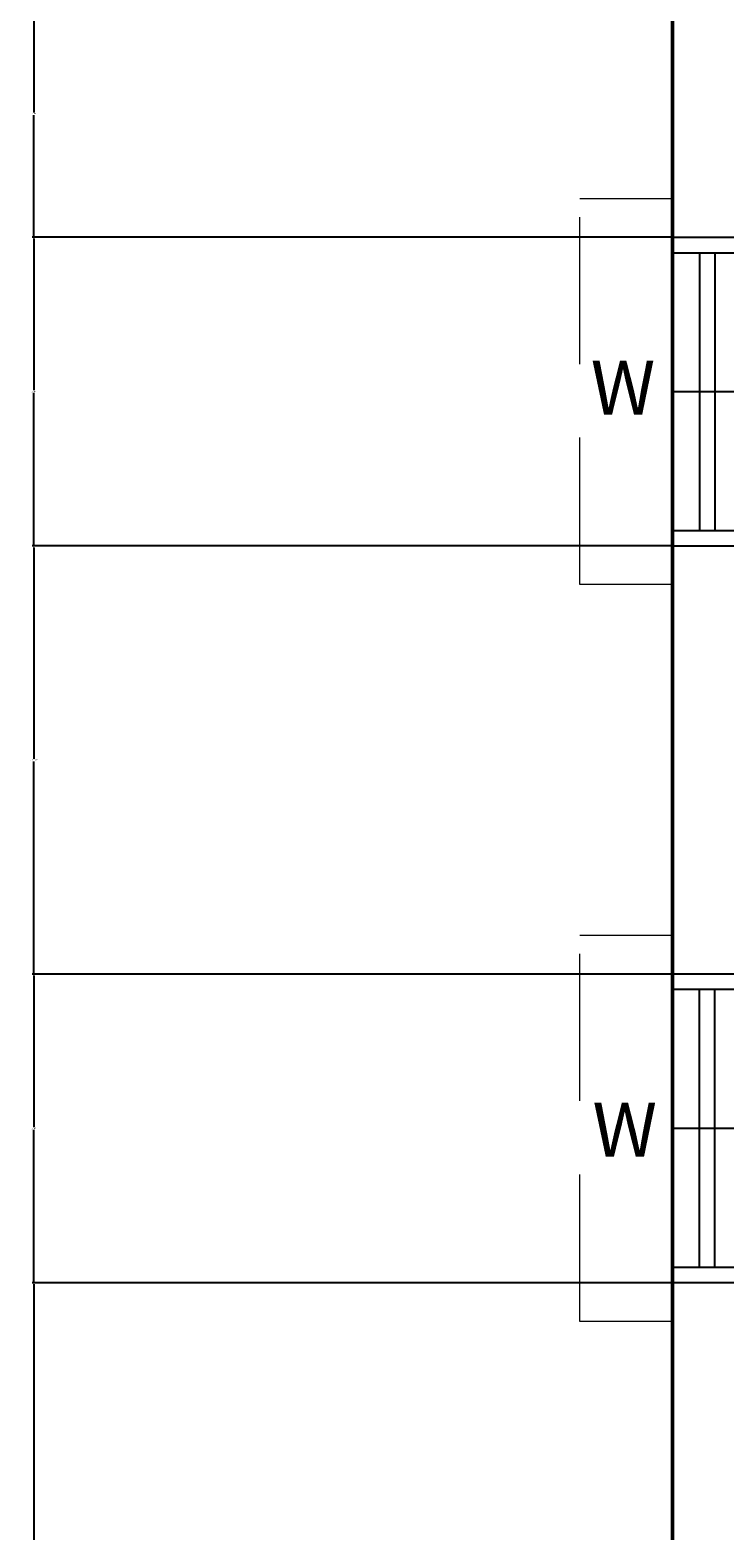
# Model space of a CAD drawing. Units: inches. Extents: x 37 to 824, y -700 to 234.
# Tile 27 of 77: x 78 to 168, y -269 to -75. Entities that reach past the tile are written whole.
import ezdxf

# ---------------------------------------------------------------- set-up
doc = ezdxf.new("R2010")
doc.units = ezdxf.units.IN
doc.header["$MEASUREMENT"] = 0
doc.linetypes.add('DASHED', pattern=[19.05, 12.7, -6.35])
for name, color, linetype, lineweight in [('A-ANNO-DIMS', 2, 'Continuous', 18), ('A-ANNO-TEXT', 7, 'Continuous', 18), ('A-GLAZ', 4, 'Continuous', 25), ('A-ROOF-OVHD', 1, 'DASHED', 18), ('A-WALL', 2, 'Continuous', 50)]:
    doc.layers.add(name, color=color, linetype=linetype, lineweight=lineweight)
doc.styles.get("Standard").update_dxf_attribs({"font": 'arial.ttf'})
doc.dimstyles.get("Standard").update_dxf_attribs({"dimtxt": 0.18, "dimasz": 0.18, "dimexe": 0.18, "dimexo": 0.0625, "dimgap": 0.09, "dimtad": 0, "dimtih": 1, "dimtoh": 1, "dimdec": 1, "dimzin": 0, "dimdsep": 46, "dimlunit": 4, "dimtxsty": 'Standard', "dimcen": 0.09, "dimadec": 0, "dimazin": 0, "dimtfac": 1, "dimtdec": 1, "dimtofl": 0, "dimtmove": 0, "dimatfit": 3, "dimfxl": 1, "dimtolj": 1, "dimtzin": 0, "dimarcsym": 0})

# ---------------------------------------------------------------- blocks, each defined once
blk = doc.blocks.new('WIN-900')
for p, q in [((0, 9), (0, 0)), ((2, 9), (2, 0)), ((20, 9), (20, 0)), ((38, 9), (38, 0)), ((40, 9), (40, 0)), ((38, 5.5), (2, 5.5)), ((38, 3.5), (2, 3.5))]:
    blk.add_line(p, q)
blk = doc.blocks.new('*D55')
at = {"layer": 'A-ANNO-DIMS', "color": 0, "lineweight": -2, "ltscale": 0.5, "transparency": 16777216}
for p, q in [((161.01, -69.41), (78.16, -69.41)), ((78.34, -69.59), (78.34, -85.23)), ((78.34, -101.23), (78.34, -85.59)), ((161.01, -101.41), (78.16, -101.41))]:
    blk.add_line(p, q, dxfattribs=at)
at = {"layer": 'A-ANNO-DIMS', "color": 0, "ltscale": 0.5, "transparency": 16777216}
for points in [[(78.31, -69.59), (78.37, -69.59), (78.34, -69.41)], [(78.31, -101.23), (78.37, -101.23), (78.34, -101.41)]]:
    blk.add_solid(points, dxfattribs=at)
at = {"layer": 'Defpoints', "color": 0, "ltscale": 0.5, "transparency": 16777216}
for p in [(161.08, -69.41), (78.34, -101.41), (161.08, -101.41)]:
    blk.add_point(p, dxfattribs=at)
at = {"layer": 'A-ANNO-DIMS', "color": 0, "ltscale": 0.5, "transparency": 16777216, "insert": (78.34, -85.41), "char_height": 0.18, "attachment_point": 5}
blk.add_mtext('\\A1;2\'-8"', dxfattribs=at)
blk = doc.blocks.new('*D56')
at = {"layer": 'A-ANNO-DIMS', "color": 0, "lineweight": -2, "ltscale": 0.5, "transparency": 16777216}
for p, q in [((161.01, -101.41), (78.16, -101.41)), ((78.34, -101.59), (78.34, -121.23)), ((78.34, -141.23), (78.34, -121.59)), ((161.01, -141.41), (78.16, -141.41))]:
    blk.add_line(p, q, dxfattribs=at)
at = {"layer": 'A-ANNO-DIMS', "color": 0, "ltscale": 0.5, "transparency": 16777216}
for points in [[(78.31, -101.59), (78.37, -101.59), (78.34, -101.41)], [(78.31, -141.23), (78.37, -141.23), (78.34, -141.41)]]:
    blk.add_solid(points, dxfattribs=at)
at = {"layer": 'Defpoints', "color": 0, "ltscale": 0.5, "transparency": 16777216}
for p in [(161.08, -101.41), (78.34, -141.41), (161.08, -141.41)]:
    blk.add_point(p, dxfattribs=at)
at = {"layer": 'A-ANNO-DIMS', "color": 0, "ltscale": 0.5, "transparency": 16777216, "insert": (78.34, -121.41), "char_height": 0.18, "attachment_point": 5}
blk.add_mtext('\\A1;3\'-4"', dxfattribs=at)
blk = doc.blocks.new('*D57')
at = {"layer": 'A-ANNO-DIMS', "color": 0, "lineweight": -2, "ltscale": 0.5, "transparency": 16777216}
for p, q in [((161.01, -141.41), (78.16, -141.41)), ((78.34, -141.59), (78.34, -168.98)), ((78.34, -196.73), (78.34, -169.34)), ((161.01, -196.91), (78.16, -196.91))]:
    blk.add_line(p, q, dxfattribs=at)
at = {"layer": 'A-ANNO-DIMS', "color": 0, "ltscale": 0.5, "transparency": 16777216}
for points in [[(78.31, -141.59), (78.37, -141.59), (78.34, -141.41)], [(78.31, -196.73), (78.37, -196.73), (78.34, -196.91)]]:
    blk.add_solid(points, dxfattribs=at)
at = {"layer": 'Defpoints', "color": 0, "ltscale": 0.5, "transparency": 16777216}
for p in [(161.08, -141.41), (78.34, -196.91), (161.08, -196.91)]:
    blk.add_point(p, dxfattribs=at)
at = {"layer": 'A-ANNO-DIMS', "color": 0, "ltscale": 0.5, "transparency": 16777216, "insert": (78.34, -169.16), "char_height": 0.18, "attachment_point": 5}
blk.add_mtext('\\A1;4\'-7 1/2"', dxfattribs=at)
blk = doc.blocks.new('*D58')
at = {"layer": 'A-ANNO-DIMS', "color": 0, "lineweight": -2, "ltscale": 0.5, "transparency": 16777216}
for p, q in [((161.01, -196.91), (78.16, -196.91)), ((78.34, -197.09), (78.34, -216.73)), ((78.34, -236.73), (78.34, -217.09)), ((161.01, -236.91), (78.16, -236.91))]:
    blk.add_line(p, q, dxfattribs=at)
at = {"layer": 'A-ANNO-DIMS', "color": 0, "ltscale": 0.5, "transparency": 16777216}
for points in [[(78.31, -197.09), (78.37, -197.09), (78.34, -196.91)], [(78.31, -236.73), (78.37, -236.73), (78.34, -236.91)]]:
    blk.add_solid(points, dxfattribs=at)
at = {"layer": 'Defpoints', "color": 0, "ltscale": 0.5, "transparency": 16777216}
for p in [(161.08, -196.91), (78.34, -236.91), (161.08, -236.91)]:
    blk.add_point(p, dxfattribs=at)
at = {"layer": 'A-ANNO-DIMS', "color": 0, "ltscale": 0.5, "transparency": 16777216, "insert": (78.34, -216.91), "char_height": 0.18, "attachment_point": 5}
blk.add_mtext('\\A1;3\'-4"', dxfattribs=at)
blk = doc.blocks.new('*D59')
at = {"layer": 'A-ANNO-DIMS', "color": 0, "lineweight": -2, "ltscale": 0.5, "transparency": 16777216}
for p, q in [((161.01, -236.91), (78.16, -236.91)), ((78.34, -237.09), (78.34, -301.23)), ((78.34, -365.73), (78.34, -301.59)), ((161.01, -365.91), (78.16, -365.91))]:
    blk.add_line(p, q, dxfattribs=at)
at = {"layer": 'A-ANNO-DIMS', "color": 0, "ltscale": 0.5, "transparency": 16777216}
for points in [[(78.31, -237.09), (78.37, -237.09), (78.34, -236.91)], [(78.31, -365.73), (78.37, -365.73), (78.34, -365.91)]]:
    blk.add_solid(points, dxfattribs=at)
at = {"layer": 'Defpoints', "color": 0, "ltscale": 0.5, "transparency": 16777216}
for p in [(161.08, -236.91), (78.34, -365.91), (161.08, -365.91)]:
    blk.add_point(p, dxfattribs=at)
at = {"layer": 'A-ANNO-DIMS', "color": 0, "ltscale": 0.5, "transparency": 16777216, "insert": (78.34, -301.41), "char_height": 0.18, "attachment_point": 5}
blk.add_mtext('\\A1;10\'-9"', dxfattribs=at)

msp = doc.modelspace()

# ---------------------------------------------------------------- linework, layer by layer
at = {"layer": 'A-ROOF-OVHD', "ltscale": 1.5}
for p, q in [((161.08, -96.41), (149.08, -96.41)), ((149.08, -146.41), (149.08, -96.41)), ((161.08, -101.41), (161.08, -96.41)), ((161.08, -141.41), (161.08, -146.41)), ((161.08, -146.41), (149.08, -146.41)), ((161.08, -191.91), (149.08, -191.91)), ((149.08, -241.91), (149.08, -191.91)), ((161.08, -196.91), (161.08, -191.91)), ((161.08, -236.91), (161.08, -241.91)), ((161.08, -241.91), (149.08, -241.91))]:
    msp.add_line(p, q, dxfattribs=at)
at = {"layer": 'A-WALL'}
msp.add_line((161.08, 75.09), (161.08, -365.91), dxfattribs=at)

# ---------------------------------------------------------------- block references
at = {"layer": 'A-GLAZ'}
for p, rotation in [((170.08, -141.41), 89.99999999999991), ((161.08, -196.91), 269.9999999999999)]:
    msp.add_blockref('WIN-900', p, dxfattribs=dict(at, rotation=rotation))

# ---------------------------------------------------------------- texts
at = {"layer": 'A-ANNO-TEXT'}
for p in [(150.49, -124.38), (150.72, -220.57)]:
    msp.add_text('W', height=7, dxfattribs=at).set_placement(p)

# ---------------------------------------------------------------- dimensions: what is measured, and where the dimension line sits
at = {"layer": 'A-ANNO-DIMS', "ltscale": 0.5}
for base, p1, p2, picture, middle in [((78.34, -101.41), (161.08, -69.41), (161.08, -101.41), '*D55', (78.34, -85.41)), ((78.34, -141.41), (161.08, -101.41), (161.08, -141.41), '*D56', (78.34, -121.41)), ((78.34, -196.91), (161.08, -141.41), (161.08, -196.91), '*D57', (78.34, -169.16)), ((78.34, -236.91), (161.08, -196.91), (161.08, -236.91), '*D58', (78.34, -216.91)), ((78.34, -365.91), (161.08, -236.91), (161.08, -365.91), '*D59', (78.34, -301.41))]:
    dim = msp.add_linear_dim(base=base, p1=p1, p2=p2, angle=90, dimstyle='Standard', override={"dimdec": 1, "dimlfac": 1, "dimrnd": 0, "dimzin": 1, "dimdsep": 46, "dimlunit": 4, "dimfrac": 2}, dxfattribs=at)
    dim.commit()
    dim.dimension.update_dxf_attribs({"geometry": picture, "text_midpoint": middle})

doc.saveas('drawing.dxf')
